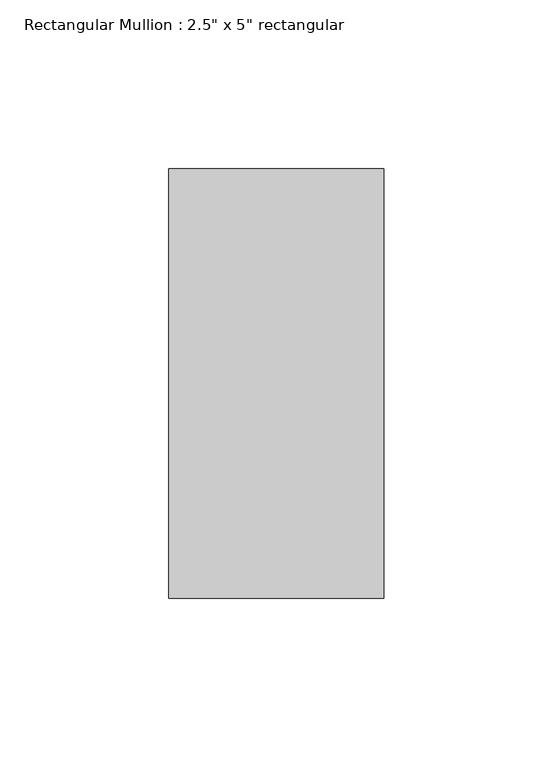
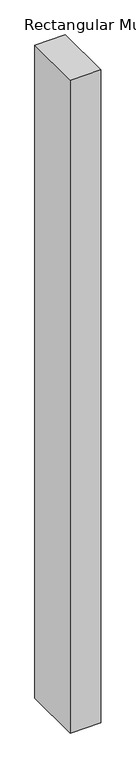
"""IFC4 building model written with IfcOpenShell, lengths in millimetres: member geometry."""

from ifc_helpers import new_model, si_unit, frame, origin, place, context, project, spatial, polyline, outline, extrude, source, transform, mapped, element, save


def member_5b6a755a(model_context):
    return source(origin(), model_context, "Body", "SweptSolid", [
        extrude(outline(polyline([(0.0, 63.5), (0.0, -63.5), (-63.5, -63.5), (-63.5, 63.5), (0.0, 63.5)])), frame((0.0, 0.0, -1433.7701004), z_axis=(0.0, 0.0, 1.0), x_axis=(1.0, 0.0, 0.0)), (0.0, 0.0, 1.0), 1433.7701004),
    ])


if __name__ == "__main__":
    model = new_model("IFC4")
    model_context = context("Model", 3, world=origin())
    ifc_project = project(units=[si_unit("LENGTHUNIT", "METRE", prefix="MILLI")], contexts=[model_context])
    site = spatial("IfcSite", under=ifc_project)
    building = spatial("IfcBuilding", under=site)
    placement = place(None, origin())
    member_shape = member_5b6a755a(model_context)
    element("IfcMember", 1, ObjectType="Rectangular Mullion : 2.5\" x 5\" rectangular", at=placement, inside=building, context=model_context, shape_type="MappedRepresentation", body=[
        mapped(member_shape, transform((0.0, 0.0, 0.0), x_axis=(1.0, 0.0, 0.0), y_axis=(0.0, 1.0, 0.0), z_axis=(0.0, 0.0, 1.0))),
    ])
    save(model, "model.ifc")

# Revit data of these elements
# Type "Rectangular Mullion : 2.5\" x 5\" rectangular"
#   built-in parameter 1007304 = 0.416667 (stored number, unit not read)
#   built-in parameter 1007301 = 0.104167 (stored number, unit not read)
#   built-in parameter 1007300 = 0.104167 (stored number, unit not read)
# Element 1 (IfcMember, "Rectangular Mullion : 2.5\" x 5\" rectangular")
#   Materials on its faces: "Aluminum"
# Materials
#   "Aluminum": class "Metal", colour RGB 247 247 247, transparency 0, Description = "Aluminum 6061", Cost = 0
